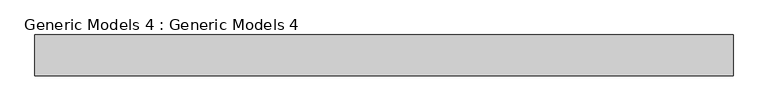
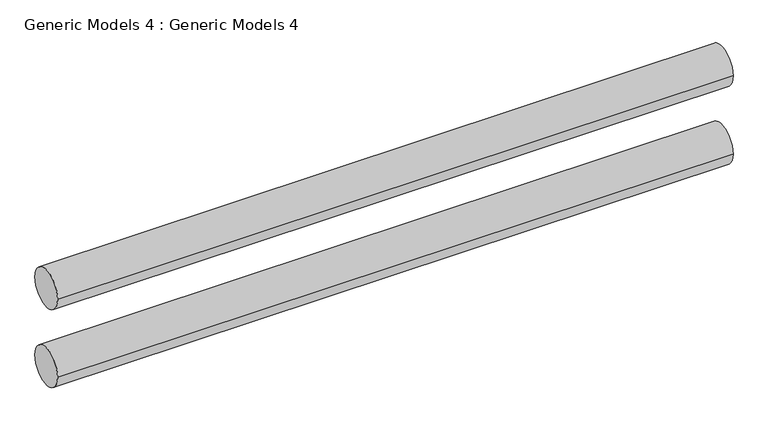
"""IFC4 building model written with IfcOpenShell, lengths in millimetres: proxy geometry, Generic Models 4 : Generic Models 4."""

from ifc_helpers import new_model, si_unit, point, frame, frame_2d, origin, place, context, project, spatial, circle_curve, trimmed, segment, composite_curve, outline, extrude, source, transform, mapped, element, save


def generic_models_4_generic_models_4_816b7f5e(model_context):
    return source(origin(), model_context, "Body", "SweptSolid", [
        extrude(outline(composite_curve([segment(trimmed(circle_curve(frame_2d((-8613.8273552, 10711.8758493)), 127.0), [point((-8740.8273552, 10711.8758493))], [point((-8486.8273552, 10711.8758493))], False, "CARTESIAN"), True, "CONTINUOUS"), segment(trimmed(circle_curve(frame_2d((-8613.8273552, 10711.8758493)), 127.0), [point((-8486.8273552, 10711.8758493))], [point((-8740.8273552, 10711.8758493))], False, "CARTESIAN"), True, "CONTINUOUS")], self_intersect=False)), frame((-6589.2415084, 0.0, 0.0), z_axis=(1.0, 0.0, 0.0), x_axis=(0.0, 1.0, 0.0)), (0.0, 0.0, 1.0), 4359.275),
        extrude(outline(composite_curve([segment(trimmed(circle_curve(frame_2d((-8613.8273552, 10178.4758493)), 127.0), [point((-8740.8273552, 10178.4758493))], [point((-8486.8273552, 10178.4758493))], False, "CARTESIAN"), True, "CONTINUOUS"), segment(trimmed(circle_curve(frame_2d((-8613.8273552, 10178.4758493)), 127.0), [point((-8486.8273552, 10178.4758493))], [point((-8740.8273552, 10178.4758493))], False, "CARTESIAN"), True, "CONTINUOUS")], self_intersect=False)), frame((-6589.2415084, 0.0, 0.0), z_axis=(1.0, 0.0, 0.0), x_axis=(0.0, 1.0, 0.0)), (0.0, 0.0, 1.0), 4359.275),
    ])


if __name__ == "__main__":
    model = new_model("IFC4")
    model_context = context("Model", 3, world=origin())
    ifc_project = project(units=[si_unit("LENGTHUNIT", "METRE", prefix="MILLI")], contexts=[model_context])
    site = spatial("IfcSite", under=ifc_project)
    building = spatial("IfcBuilding", under=site)
    placement = place(None, origin())
    generic_models_4_generic_models_4_shape = generic_models_4_generic_models_4_816b7f5e(model_context)
    element("IfcBuildingElementProxy", 1, Name="Generic Models 4 : Generic Models 4", ObjectType="Generic Models 4 : Generic Models 4", at=placement, inside=building, context=model_context, shape_type="MappedRepresentation", body=[
        mapped(generic_models_4_generic_models_4_shape, transform((0.0, 0.0, 0.0), x_axis=(1.0, 0.0, 0.0), y_axis=(0.0, 1.0, 0.0), z_axis=(0.0, 0.0, 1.0))),
    ])
    save(model, "model.ifc")

# Revit data of these elements
# Element 1 (IfcBuildingElementProxy, "Generic Models 4 : Generic Models 4")
#   Materials on its faces: "Brick, Soldier Course"
# Materials
#   "Brick, Soldier Course": class "Masonry", colour RGB 170 98 104, transparency 0, Description = "Common brick soldier coursed", Cost = 0
